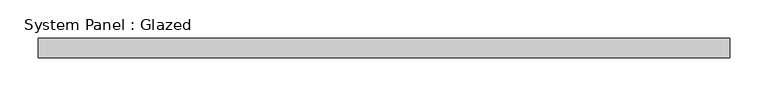
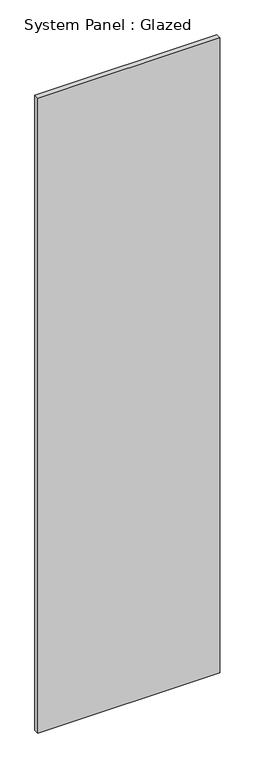
"""IFC4 building model written with IfcOpenShell, lengths in millimetres: plate geometry, System Panel : Glazed."""

from ifc_helpers import new_model, si_unit, origin, origin_with_axes, place, context, project, spatial, polyline, outline, extrude, source, transform, mapped, element, save


def system_panel_glazed_51964df0(model_context):
    return source(origin(), model_context, "Body", "SweptSolid", [
        extrude(outline(polyline([(450.85, 19.05), (-450.85, 19.05), (-450.85, 44.45), (450.85, 44.45), (450.85, 19.05)])), origin_with_axes(), (0.0, 0.0, 1.0), 3327.61006),
    ])


if __name__ == "__main__":
    model = new_model("IFC4")
    model_context = context("Model", 3, world=origin())
    ifc_project = project(units=[si_unit("LENGTHUNIT", "METRE", prefix="MILLI")], contexts=[model_context])
    site = spatial("IfcSite", under=ifc_project)
    building = spatial("IfcBuilding", under=site)
    placement = place(None, origin())
    system_panel_glazed_shape = system_panel_glazed_51964df0(model_context)
    element("IfcPlate", 1, ObjectType="System Panel : Glazed", at=placement, inside=building, context=model_context, shape_type="MappedRepresentation", body=[
        mapped(system_panel_glazed_shape, transform((0.0, 0.0, 0.0), x_axis=(1.0, 0.0, 0.0), y_axis=(0.0, 1.0, 0.0), z_axis=(0.0, 0.0, 1.0))),
    ])
    save(model, "model.ifc")

# Revit data of these elements
# Type "System Panel : Glazed"
#   Construction Type Id = "GSP4R"
#   Analytic Construction = "1/8 in Pilkington single glazing"
#   Visual Light Transmittance = 0.9
#   Solar Heat Gain Coefficient = 0.86
#   Heat Transfer Coefficient (U) = 1.18115 BTU/(h·ft²·°F)
#   Define Thermal Properties by = 1
# Element 1 (IfcPlate, "System Panel : Glazed")
#   Materials on its faces: "Glass"
# Materials
#   "Glass": class "Glass", colour RGB 0 128 192, transparency 0.75, Description = "Soda Lime Glass", Cost = 0
